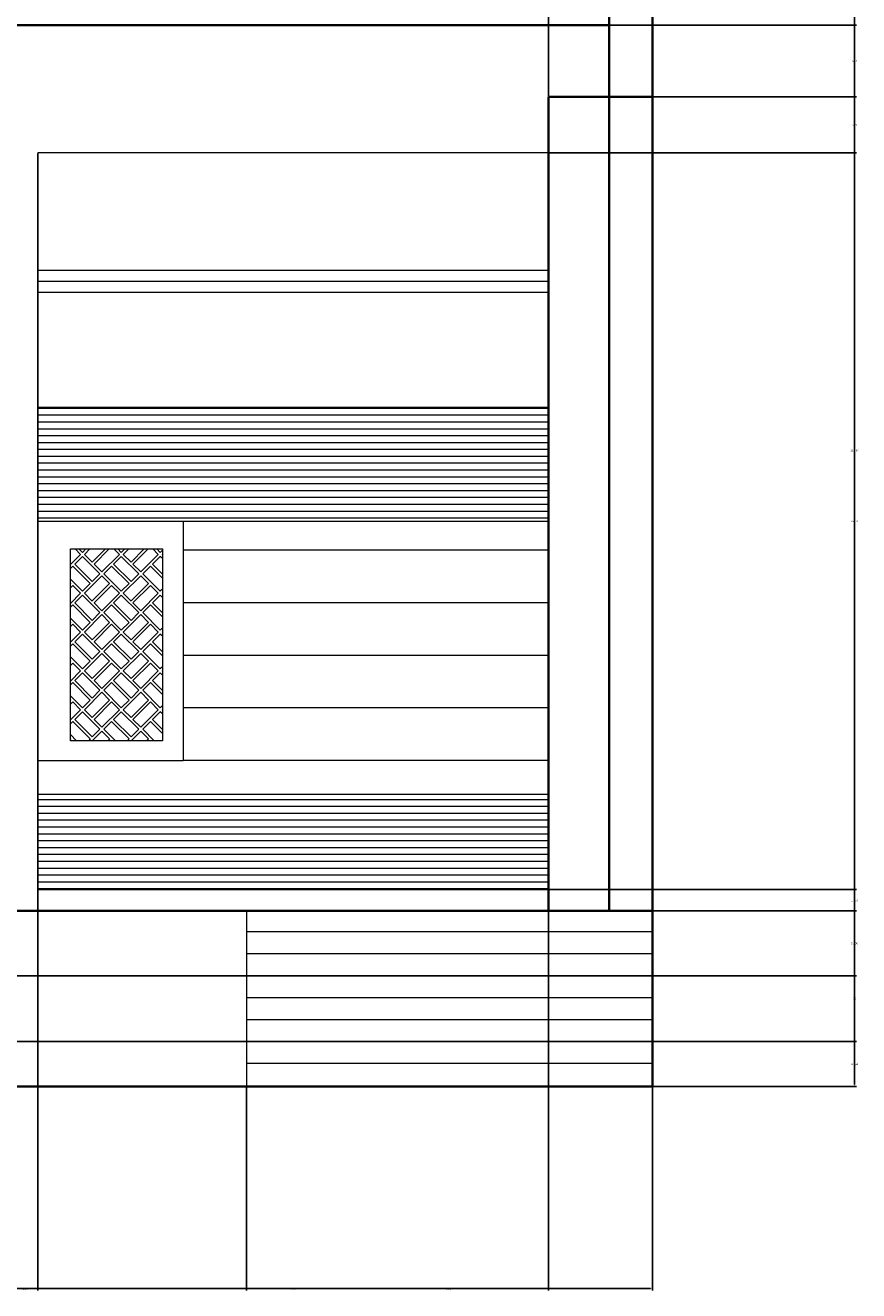
# Model space of a CAD drawing. Units: inches. Extents: x -7 to 391, y -12 to 303.
# Tile 4 of 5: x 315 to 391, y -12 to 103. Entities that reach past the tile are written whole.
import ezdxf

# ---------------------------------------------------------------- set-up
doc = ezdxf.new("R2010")
doc.units = ezdxf.units.IN
doc.header["$MEASUREMENT"] = 0
for name, color, linetype, lineweight in [('A-ANNO-DIMS', 2, 'Continuous', 18), ('A-DOOR', 3, 'Continuous', 18), ('A-ELEV', 7, 'Continuous', 35), ('A-ELEV-PATT', 8, 'Continuous', 13), ('A-FLOR-STRS', 2, 'Continuous', 18)]:
    doc.layers.add(name, color=color, linetype=linetype, lineweight=lineweight)
doc.styles.get("Standard").update_dxf_attribs({"font": 'arial.ttf'})
doc.dimstyles.get("Standard").update_dxf_attribs({"dimtxt": 0.18, "dimasz": 0.18, "dimexe": 0.18, "dimexo": 0.0625, "dimgap": 0.09, "dimtad": 0, "dimtih": 1, "dimtoh": 1, "dimdec": 4, "dimzin": 0, "dimdsep": 46, "dimtxsty": 'Standard', "dimcen": 0.09, "dimadec": 0, "dimazin": 0, "dimtfac": 1, "dimtdec": 4, "dimtofl": 0, "dimtmove": 0, "dimatfit": 3, "dimfxl": 1, "dimtolj": 1, "dimtzin": 0, "dimarcsym": 0})

# ---------------------------------------------------------------- blocks, each defined once
blk = doc.blocks.new('*D1')
at = {"layer": 'A-ANNO-DIMS', "color": 0, "lineweight": -2, "transparency": 16777216}
for p, q in [((372.08, 122.18), (390.6, 122.18)), ((390.42, 122), (390.42, 64.44)), ((390.42, 6.53), (390.42, 64.08)), ((150.31, 6.35), (390.6, 6.35))]:
    blk.add_line(p, q, dxfattribs=at)
at = {"layer": 'A-ANNO-DIMS', "color": 0, "transparency": 16777216}
for points in [[(390.39, 122), (390.45, 122), (390.42, 122.18)], [(390.39, 6.53), (390.45, 6.53), (390.42, 6.35)]]:
    blk.add_solid(points, dxfattribs=at)
at = {"layer": 'Defpoints', "color": 0, "transparency": 16777216}
for p in [(372.02, 122.18), (390.42, 122.18), (150.24, 6.35)]:
    blk.add_point(p, dxfattribs=at)
at = {"layer": 'A-ANNO-DIMS', "color": 0, "transparency": 16777216, "insert": (390.42, 64.26), "char_height": 0.18, "attachment_point": 5}
blk.add_mtext('\\A1;115.83', dxfattribs=at)
blk = doc.blocks.new('*D39')
at = {"layer": 'A-ANNO-DIMS', "color": 0, "lineweight": -2, "transparency": 16777216}
for p, q in [((372.02, 154.28), (372.02, -12.23)), ((246.74, 6.28), (246.74, -12.23)), ((246.92, -12.05), (308.92, -12.05)), ((371.84, -12.05), (309.84, -12.05))]:
    blk.add_line(p, q, dxfattribs=at)
at = {"layer": 'A-ANNO-DIMS', "color": 0, "transparency": 16777216}
for points in [[(246.92, -12.02), (246.92, -12.08), (246.74, -12.05)], [(371.84, -12.02), (371.84, -12.08), (372.02, -12.05)]]:
    blk.add_solid(points, dxfattribs=at)
at = {"layer": 'Defpoints', "color": 0, "transparency": 16777216}
for p in [(372.02, 154.35), (246.74, 6.35), (372.02, -12.05)]:
    blk.add_point(p, dxfattribs=at)
at = {"layer": 'A-ANNO-DIMS', "color": 0, "transparency": 16777216, "insert": (309.38, -12.05), "char_height": 0.18, "attachment_point": 5}
blk.add_mtext('\\A1;125.28', dxfattribs=at)
blk = doc.blocks.new('*D41')
at = {"layer": 'A-ANNO-DIMS', "color": 0, "lineweight": -2, "transparency": 16777216}
for p, q in [((283.68, 6.28), (283.68, -12.23)), ((335.08, 6.28), (335.08, -12.23)), ((283.86, -12.05), (309.06, -12.05)), ((334.9, -12.05), (309.7, -12.05))]:
    blk.add_line(p, q, dxfattribs=at)
at = {"layer": 'A-ANNO-DIMS', "color": 0, "transparency": 16777216}
for points in [[(283.86, -12.02), (283.86, -12.08), (283.68, -12.05)], [(334.9, -12.02), (334.9, -12.08), (335.08, -12.05)]]:
    blk.add_solid(points, dxfattribs=at)
at = {"layer": 'Defpoints', "color": 0, "transparency": 16777216}
for p in [(283.68, 6.35), (335.08, 6.35), (335.08, -12.05)]:
    blk.add_point(p, dxfattribs=at)
at = {"layer": 'A-ANNO-DIMS', "color": 0, "transparency": 16777216, "insert": (309.38, -12.05), "char_height": 0.18, "attachment_point": 5}
blk.add_mtext('\\A1;51.4', dxfattribs=at)
blk = doc.blocks.new('*D42')
at = {"layer": 'A-ANNO-DIMS', "color": 0, "lineweight": -2, "transparency": 16777216}
for p, q in [((335.08, 6.28), (335.08, -12.23)), ((372.02, 6.28), (372.02, -12.23)), ((335.26, -12.05), (353.16, -12.05)), ((371.84, -12.05), (353.94, -12.05))]:
    blk.add_line(p, q, dxfattribs=at)
at = {"layer": 'A-ANNO-DIMS', "color": 0, "transparency": 16777216}
for points in [[(335.26, -12.02), (335.26, -12.08), (335.08, -12.05)], [(371.84, -12.02), (371.84, -12.08), (372.02, -12.05)]]:
    blk.add_solid(points, dxfattribs=at)
at = {"layer": 'Defpoints', "color": 0, "transparency": 16777216}
for p in [(335.08, 6.35), (372.02, 6.35), (372.02, -12.05)]:
    blk.add_point(p, dxfattribs=at)
at = {"layer": 'A-ANNO-DIMS', "color": 0, "transparency": 16777216, "insert": (353.55, -12.05), "char_height": 0.18, "attachment_point": 5}
blk.add_mtext('\\A1;36.94', dxfattribs=at)
blk = doc.blocks.new('*D49')
at = {"layer": 'A-ANNO-DIMS', "color": 0, "lineweight": -2, "transparency": 16777216}
for p, q in [((313.81, 91.3), (313.81, -12.23)), ((316.08, 91.3), (316.08, -12.23)), ((313.99, -12.05), (314.62, -12.05)), ((315.9, -12.05), (315.27, -12.05))]:
    blk.add_line(p, q, dxfattribs=at)
at = {"layer": 'A-ANNO-DIMS', "color": 0, "transparency": 16777216}
for points in [[(313.99, -12.02), (313.99, -12.08), (313.81, -12.05)], [(315.9, -12.02), (315.9, -12.08), (316.08, -12.05)]]:
    blk.add_solid(points, dxfattribs=at)
at = {"layer": 'Defpoints', "color": 0, "transparency": 16777216}
for p in [(313.81, 91.37), (316.08, 91.37), (316.08, -12.05)]:
    blk.add_point(p, dxfattribs=at)
at = {"layer": 'A-ANNO-DIMS', "color": 0, "transparency": 16777216, "insert": (314.94, -12.05), "char_height": 0.18, "attachment_point": 5}
blk.add_mtext('\\A1;2.27', dxfattribs=at)
blk = doc.blocks.new('*D50')
at = {"layer": 'A-ANNO-DIMS', "color": 0, "lineweight": -2, "transparency": 16777216}
for p, q in [((316.08, 91.3), (316.08, -12.23)), ((362.55, 91.3), (362.55, -12.23)), ((316.26, -12.05), (338.92, -12.05)), ((362.37, -12.05), (339.71, -12.05))]:
    blk.add_line(p, q, dxfattribs=at)
at = {"layer": 'A-ANNO-DIMS', "color": 0, "transparency": 16777216}
for points in [[(316.26, -12.02), (316.26, -12.08), (316.08, -12.05)], [(362.37, -12.02), (362.37, -12.08), (362.55, -12.05)]]:
    blk.add_solid(points, dxfattribs=at)
at = {"layer": 'Defpoints', "color": 0, "transparency": 16777216}
for p in [(316.08, 91.37), (362.55, 91.37), (362.55, -12.05)]:
    blk.add_point(p, dxfattribs=at)
at = {"layer": 'A-ANNO-DIMS', "color": 0, "transparency": 16777216, "insert": (339.31, -12.05), "char_height": 0.18, "attachment_point": 5}
blk.add_mtext('\\A1;46.47', dxfattribs=at)
blk = doc.blocks.new('*D51')
at = {"layer": 'A-ANNO-DIMS', "color": 0, "lineweight": -2, "transparency": 16777216}
for p, q in [((362.55, 96.52), (362.55, 303.01)), ((368.1, 103.04), (368.1, 303.01)), ((362.73, 302.83), (364.93, 302.83)), ((367.92, 302.83), (365.72, 302.83))]:
    blk.add_line(p, q, dxfattribs=at)
at = {"layer": 'A-ANNO-DIMS', "color": 0, "transparency": 16777216}
for points in [[(362.73, 302.86), (362.73, 302.8), (362.55, 302.83)], [(367.92, 302.86), (367.92, 302.8), (368.1, 302.83)]]:
    blk.add_solid(points, dxfattribs=at)
at = {"layer": 'Defpoints', "color": 0, "transparency": 16777216}
for p in [(368.1, 302.83), (368.1, 102.98), (362.55, 96.46)]:
    blk.add_point(p, dxfattribs=at)
at = {"layer": 'A-ANNO-DIMS', "color": 0, "transparency": 16777216, "insert": (365.32, 302.83), "char_height": 0.18, "attachment_point": 5}
blk.add_mtext('\\A1;5.549', dxfattribs=at)
blk = doc.blocks.new('*D57')
at = {"layer": 'A-ANNO-DIMS', "color": 0, "lineweight": -2, "transparency": 16777216}
for p, q in [((372.08, 22.35), (390.6, 22.35)), ((390.42, 22.17), (390.42, 14.53)), ((390.42, 6.53), (390.42, 14.16)), ((372.08, 6.35), (390.6, 6.35))]:
    blk.add_line(p, q, dxfattribs=at)
at = {"layer": 'A-ANNO-DIMS', "color": 0, "transparency": 16777216}
for points in [[(390.39, 22.17), (390.45, 22.17), (390.42, 22.35)], [(390.39, 6.53), (390.45, 6.53), (390.42, 6.35)]]:
    blk.add_solid(points, dxfattribs=at)
at = {"layer": 'Defpoints', "color": 0, "transparency": 16777216}
for p in [(372.02, 22.35), (390.42, 22.35), (372.02, 6.35)]:
    blk.add_point(p, dxfattribs=at)
at = {"layer": 'A-ANNO-DIMS', "color": 0, "transparency": 16777216, "insert": (390.42, 14.35), "char_height": 0.18, "attachment_point": 5}
blk.add_mtext('\\A1;16', dxfattribs=at)
blk = doc.blocks.new('*D58')
at = {"layer": 'A-ANNO-DIMS', "color": 0, "lineweight": -2, "transparency": 16777216}
for p, q in [((362.61, 24.3), (390.6, 24.3)), ((390.42, 24.12), (390.42, 23.5)), ((390.42, 22.53), (390.42, 23.14)), ((372.08, 22.35), (390.6, 22.35))]:
    blk.add_line(p, q, dxfattribs=at)
at = {"layer": 'A-ANNO-DIMS', "color": 0, "transparency": 16777216}
for points in [[(390.39, 24.12), (390.45, 24.12), (390.42, 24.3)], [(390.39, 22.53), (390.45, 22.53), (390.42, 22.35)]]:
    blk.add_solid(points, dxfattribs=at)
at = {"layer": 'Defpoints', "color": 0, "transparency": 16777216}
for p in [(362.55, 24.3), (390.42, 24.3), (372.02, 22.35)]:
    blk.add_point(p, dxfattribs=at)
at = {"layer": 'A-ANNO-DIMS', "color": 0, "transparency": 16777216, "insert": (390.42, 23.32), "char_height": 0.18, "attachment_point": 5}
blk.add_mtext('\\A1;1.952', dxfattribs=at)
blk = doc.blocks.new('*D59')
at = {"layer": 'A-ANNO-DIMS', "color": 0, "lineweight": -2, "transparency": 16777216}
for p, q in [((362.61, 91.37), (390.6, 91.37)), ((390.42, 91.19), (390.42, 58.01)), ((390.42, 24.48), (390.42, 57.65)), ((362.61, 24.3), (390.6, 24.3))]:
    blk.add_line(p, q, dxfattribs=at)
at = {"layer": 'A-ANNO-DIMS', "color": 0, "transparency": 16777216}
for points in [[(390.39, 91.19), (390.45, 91.19), (390.42, 91.37)], [(390.39, 24.48), (390.45, 24.48), (390.42, 24.3)]]:
    blk.add_solid(points, dxfattribs=at)
at = {"layer": 'Defpoints', "color": 0, "transparency": 16777216}
for p in [(362.55, 91.37), (390.42, 91.37), (362.55, 24.3)]:
    blk.add_point(p, dxfattribs=at)
at = {"layer": 'A-ANNO-DIMS', "color": 0, "transparency": 16777216, "insert": (390.42, 57.83), "char_height": 0.18, "attachment_point": 5}
blk.add_mtext('\\A1;67.07', dxfattribs=at)
blk = doc.blocks.new('*D60')
at = {"layer": 'A-ANNO-DIMS', "color": 0, "lineweight": -2, "transparency": 16777216}
for p, q in [((372.08, 96.46), (390.6, 96.46)), ((390.42, 96.28), (390.42, 94.09)), ((390.42, 91.55), (390.42, 93.73)), ((362.61, 91.37), (390.6, 91.37))]:
    blk.add_line(p, q, dxfattribs=at)
at = {"layer": 'A-ANNO-DIMS', "color": 0, "transparency": 16777216}
for points in [[(390.39, 96.28), (390.45, 96.28), (390.42, 96.46)], [(390.39, 91.55), (390.45, 91.55), (390.42, 91.37)]]:
    blk.add_solid(points, dxfattribs=at)
at = {"layer": 'Defpoints', "color": 0, "transparency": 16777216}
for p in [(372.02, 96.46), (390.42, 96.46), (362.55, 91.37)]:
    blk.add_point(p, dxfattribs=at)
at = {"layer": 'A-ANNO-DIMS', "color": 0, "transparency": 16777216, "insert": (390.42, 93.91), "char_height": 0.18, "attachment_point": 5}
blk.add_mtext('\\A1;5.09', dxfattribs=at)
blk = doc.blocks.new('*D61')
at = {"layer": 'A-ANNO-DIMS', "color": 0, "lineweight": -2, "transparency": 16777216}
for p, q in [((368.16, 102.98), (390.6, 102.98)), ((390.42, 102.8), (390.42, 99.9)), ((390.42, 96.64), (390.42, 99.53)), ((372.08, 96.46), (390.6, 96.46))]:
    blk.add_line(p, q, dxfattribs=at)
at = {"layer": 'A-ANNO-DIMS', "color": 0, "transparency": 16777216}
for points in [[(390.39, 102.8), (390.45, 102.8), (390.42, 102.98)], [(390.39, 96.64), (390.45, 96.64), (390.42, 96.46)]]:
    blk.add_solid(points, dxfattribs=at)
at = {"layer": 'Defpoints', "color": 0, "transparency": 16777216}
for p in [(368.1, 102.98), (390.42, 102.98), (372.02, 96.46)]:
    blk.add_point(p, dxfattribs=at)
at = {"layer": 'A-ANNO-DIMS', "color": 0, "transparency": 16777216, "insert": (390.42, 99.72), "char_height": 0.18, "attachment_point": 5}
blk.add_mtext('\\A1;6.52', dxfattribs=at)
blk = doc.blocks.new('*D74')
at = {"layer": 'A-ANNO-DIMS', "color": 0, "lineweight": -2, "transparency": 16777216}
for p, q in [((283.74, 10.44), (390.6, 10.44)), ((390.42, 10.26), (390.42, 8.57)), ((390.42, 6.53), (390.42, 8.21)), ((283.74, 6.35), (390.6, 6.35))]:
    blk.add_line(p, q, dxfattribs=at)
at = {"layer": 'A-ANNO-DIMS', "color": 0, "transparency": 16777216}
for points in [[(390.39, 10.26), (390.45, 10.26), (390.42, 10.44)], [(390.39, 6.53), (390.45, 6.53), (390.42, 6.35)]]:
    blk.add_solid(points, dxfattribs=at)
at = {"layer": 'Defpoints', "color": 0, "transparency": 16777216}
for p in [(283.68, 10.44), (390.42, 10.44), (283.68, 6.35)]:
    blk.add_point(p, dxfattribs=at)
at = {"layer": 'A-ANNO-DIMS', "color": 0, "transparency": 16777216, "insert": (390.42, 8.39), "char_height": 0.18, "attachment_point": 5}
blk.add_mtext('\\A1;4.094', dxfattribs=at)
blk = doc.blocks.new('*D75')
at = {"layer": 'A-ANNO-DIMS', "color": 0, "lineweight": -2, "transparency": 16777216}
for p, q in [((283.74, 16.44), (390.6, 16.44)), ((390.42, 16.26), (390.42, 13.62)), ((390.42, 10.62), (390.42, 13.26)), ((283.74, 10.44), (390.6, 10.44))]:
    blk.add_line(p, q, dxfattribs=at)
at = {"layer": 'A-ANNO-DIMS', "color": 0, "transparency": 16777216}
for points in [[(390.39, 16.26), (390.45, 16.26), (390.42, 16.44)], [(390.39, 10.62), (390.45, 10.62), (390.42, 10.44)]]:
    blk.add_solid(points, dxfattribs=at)
at = {"layer": 'Defpoints', "color": 0, "transparency": 16777216}
for p in [(283.68, 16.44), (390.42, 16.44), (283.68, 10.44)]:
    blk.add_point(p, dxfattribs=at)
at = {"layer": 'A-ANNO-DIMS', "color": 0, "transparency": 16777216, "insert": (390.42, 13.44), "char_height": 0.18, "attachment_point": 5}
blk.add_mtext('\\A1;6', dxfattribs=at)
blk = doc.blocks.new('*D76')
at = {"layer": 'A-ANNO-DIMS', "color": 0, "lineweight": -2, "transparency": 16777216}
for p, q in [((283.74, 22.35), (390.6, 22.35)), ((390.42, 22.17), (390.42, 19.57)), ((390.42, 16.62), (390.42, 19.21)), ((283.74, 16.44), (390.6, 16.44))]:
    blk.add_line(p, q, dxfattribs=at)
at = {"layer": 'A-ANNO-DIMS', "color": 0, "transparency": 16777216}
for points in [[(390.39, 22.17), (390.45, 22.17), (390.42, 22.35)], [(390.39, 16.62), (390.45, 16.62), (390.42, 16.44)]]:
    blk.add_solid(points, dxfattribs=at)
at = {"layer": 'Defpoints', "color": 0, "transparency": 16777216}
for p in [(283.68, 22.35), (390.42, 22.35), (283.68, 16.44)]:
    blk.add_point(p, dxfattribs=at)
at = {"layer": 'A-ANNO-DIMS', "color": 0, "transparency": 16777216, "insert": (390.42, 19.39), "char_height": 0.18, "attachment_point": 5}
blk.add_mtext('\\A1;5.906', dxfattribs=at)

msp = doc.modelspace()

# ---------------------------------------------------------------- hatches: boundary and pattern name
at = {"layer": 'A-ELEV-PATT'}
h = msp.add_hatch(dxfattribs=at)
h.set_pattern_fill('ANSI31', color=256, scale=5, angle=135)
h.paths.add_polyline_path([(313.8105, 33.3417), (264.1332, 33.3417), (264.1332, 24.2974), (313.8105, 24.2974)])
h.paths.add_polyline_path([(362.5506, 32.9858), (316.076, 32.9858), (316.076, 24.2974), (362.5506, 24.2974)])
h.paths.add_polyline_path([(362.5506, 68.2193), (316.076, 68.2193), (316.076, 57.8315), (329.3009, 57.8315), (362.5506, 57.8315)])
h.paths.add_polyline_path([(313.8105, 68.2193), (264.1332, 68.2193), (264.1332, 57.8315), (313.8105, 57.8315)])
h = msp.add_hatch(dxfattribs=at)
h.set_pattern_fill('2X2µØ×©', color=256, scale=5, angle=135)
h.set_pattern_definition([(135, (0, 0), (-3.535534, 2e-16), [2.25, -0.25, 1, -0.25, 1, -0.25]), (135, (-0.707, -0.707), (-3.535534, 2e-16), [2.25, -2.75]), (135, (-0.884, -0.884), (-3.535534, 2e-16), [2.25, -2.75]), (135, (-1.591, -1.591), (-3.535534, 2e-16), [2.25, -0.25, 1, -0.25, 1, -0.25]), (225, (0, 0), (-4e-16, -3.535534), [1, -0.25, 1, -0.25, 2.25, -0.25]), (225, (-1.591, 1.591), (-4e-16, -3.535534), [1, -0.25, 1, -0.25, 2.25, -0.25]), (225, (-2.4749, 2.4749), (-4e-16, -3.535534), [2.25, -2.75]), (225, (-2.6517, 2.6517), (-4e-16, -3.535534), [2.25, -2.75])])
h.paths.add_polyline_path([(275.4815, 55.2969), (267.1041, 55.2969), (267.1041, 37.8416), (275.4815, 37.8416)])
h.paths.add_polyline_path([(327.4242, 55.2969), (319.0469, 55.2969), (319.0469, 37.8416), (327.4242, 37.8416)])

# ---------------------------------------------------------------- linework, layer by layer
at = {"layer": 'A-DOOR'}
for p, q in [((316.076, 80.6934), (362.5506, 80.6934)), ((316.076, 79.6934), (362.5506, 79.6934)), ((316.076, 79.6934), (362.5506, 79.6934)), ((316.076, 78.6934), (362.5506, 78.6934)), ((316.076, 68.2193), (362.5506, 68.2193)), ((316.076, 57.8315), (362.5506, 57.8315)), ((329.3009, 55.2077), (362.5506, 55.2077)), ((329.3009, 50.4241), (362.5506, 50.4241)), ((329.3009, 45.6405), (362.5506, 45.6405)), ((329.3009, 40.8569), (362.5506, 40.8569)), ((329.3009, 36.0733), (362.5506, 36.0733)), ((316.076, 32.9858), (362.5506, 32.9858))]:
    msp.add_line(p, q, dxfattribs=at)
for points in [[(362.5506, 91.3657), (316.076, 91.3657), (316.076, 24.2974), (362.5506, 24.2974)], [(316.076, 57.8315), (329.3009, 57.8315), (329.3009, 36.0134), (316.076, 36.0134)], [(319.0469, 55.2969), (327.4242, 55.2969), (327.4242, 37.8416), (319.0469, 37.8416)]]:
    msp.add_lwpolyline(points, close=True, dxfattribs=at)
at = {"layer": 'A-ELEV'}
for p, q in [((372.0212, 135.1767), (372.0212, 6.3452)), ((368.0993, 96.456), (368.0993, 122.1767)), ((258.2707, 102.9762), (368.0993, 102.9762)), ((362.5506, 22.3452), (362.5506, 96.456)), ((362.5506, 96.456), (368.0993, 96.456)), ((368.0993, 22.3452), (368.0993, 96.456)), ((368.0993, 96.456), (372.0212, 96.456)), ((12.0212, 22.3452), (372.0212, 22.3452)), ((12.0212, 6.3452), (372.0212, 6.3452))]:
    msp.add_line(p, q, dxfattribs=at)
at = {"layer": 'A-FLOR-STRS'}
for p, q in [((335.0799, 22.3452), (335.0799, 6.3452)), ((372.0212, 20.4396), (335.0799, 20.4396)), ((372.0212, 18.4396), (335.0799, 18.4396)), ((283.6807, 16.4396), (335.0799, 16.4396)), ((372.0212, 16.4396), (335.0799, 16.4396)), ((372.0212, 14.4396), (335.0799, 14.4396)), ((372.0212, 12.4396), (335.0799, 12.4396)), ((283.6807, 10.4396), (335.0799, 10.4396)), ((372.0212, 10.4396), (335.0799, 10.4396)), ((372.0212, 8.4396), (335.0799, 8.4396))]:
    msp.add_line(p, q, dxfattribs=at)

# ---------------------------------------------------------------- dimensions: what is measured, and where the dimension line sits
at = {"layer": 'A-ANNO-DIMS'}
for base, p1, p2, override, picture, middle in [((368.0993, 302.832), (362.5506, 96.456), (368.0993, 102.9762), {"dimdec": 3, "dimlfac": 1, "dimrnd": 0, "dimzin": 0, "dimdsep": 46, "dimlunit": 2}, '*D51', (365.325, 302.832)), ((372.0212, -12.0548), (246.7395, 6.3452), (372.0212, 154.3452), {"dimdec": 2, "dimlfac": 1, "dimrnd": 0, "dimzin": 0, "dimdsep": 46, "dimlunit": 2}, '*D39', (309.3803, -12.0548)), ((316.076, -12.0548), (313.8105, 91.3657), (316.076, 91.3657), {"dimdec": 2, "dimlfac": 1, "dimrnd": 0, "dimzin": 0, "dimdsep": 46, "dimlunit": 2}, '*D49', (314.9432, -12.0548)), ((362.5506, -12.0548), (316.076, 91.3657), (362.5506, 91.3657), {"dimdec": 2, "dimlfac": 1, "dimrnd": 0, "dimzin": 0, "dimdsep": 46, "dimlunit": 2}, '*D50', (339.3133, -12.0548)), ((335.0799, -12.0548), (283.6807, 6.3452), (335.0799, 6.3452), {"dimdec": 1, "dimlfac": 1, "dimrnd": 0, "dimzin": 0, "dimdsep": 46, "dimlunit": 2}, '*D41', (309.3803, -12.0548)), ((372.0212, -12.0548), (335.0799, 6.3452), (372.0212, 6.3452), {"dimdec": 2, "dimlfac": 1, "dimrnd": 0, "dimzin": 0, "dimdsep": 46, "dimlunit": 2}, '*D42', (353.5506, -12.0548))]:
    dim = msp.add_linear_dim(base=base, p1=p1, p2=p2, dimstyle='Standard', override=override, dxfattribs=at)
    dim.commit()
    dim.dimension.update_dxf_attribs({"geometry": picture, "text_midpoint": middle})
for base, p1, p2, override, picture, middle in [((390.4212, 122.1767), (150.2426, 6.3452), (372.0212, 122.1767), {"dimdec": 2, "dimlfac": 1, "dimrnd": 0, "dimzin": 0, "dimdsep": 46, "dimlunit": 2}, '*D1', (390.4212, 64.261)), ((390.4212, 102.9762), (372.0212, 96.456), (368.0993, 102.9762), {"dimdec": 2, "dimlfac": 1, "dimrnd": 0, "dimzin": 0, "dimdsep": 46, "dimlunit": 2}, '*D61', (390.4212, 99.7161)), ((390.4212, 96.456), (362.5506, 91.3657), (372.0212, 96.456), {"dimdec": 2, "dimlfac": 1, "dimrnd": 0, "dimzin": 0, "dimdsep": 46, "dimlunit": 2}, '*D60', (390.4212, 93.9109)), ((390.4212, 91.3657), (362.5506, 24.2974), (362.5506, 91.3657), {"dimdec": 2, "dimlfac": 1, "dimrnd": 0, "dimzin": 0, "dimdsep": 46, "dimlunit": 2}, '*D59', (390.4212, 57.8315)), ((390.4212, 24.2974), (372.0212, 22.3452), (362.5506, 24.2974), {"dimdec": 3, "dimlfac": 1, "dimrnd": 0, "dimzin": 0, "dimdsep": 46, "dimlunit": 2}, '*D58', (390.4212, 23.3213)), ((390.4212, 22.3452), (283.6807, 16.4396), (283.6807, 22.3452), {"dimdec": 3, "dimlfac": 1, "dimrnd": 0, "dimzin": 0, "dimdsep": 46, "dimlunit": 2}, '*D76', (390.4212, 19.3924)), ((390.4212, 22.3452), (372.0212, 6.3452), (372.0212, 22.3452), {"dimdec": 0, "dimlfac": 1, "dimrnd": 0, "dimzin": 0, "dimdsep": 46, "dimlunit": 2}, '*D57', (390.4212, 14.3452)), ((390.4212, 16.4396), (283.6807, 10.4396), (283.6807, 16.4396), {"dimdec": 0, "dimlfac": 1, "dimrnd": 0, "dimzin": 0, "dimdsep": 46, "dimlunit": 2}, '*D75', (390.4212, 13.4396)), ((390.4212, 10.4396), (283.6807, 6.3452), (283.6807, 10.4396), {"dimdec": 3, "dimlfac": 1, "dimrnd": 0, "dimzin": 0, "dimdsep": 46, "dimlunit": 2}, '*D74', (390.4212, 8.3924))]:
    dim = msp.add_linear_dim(base=base, p1=p1, p2=p2, angle=90, dimstyle='Standard', override=override, dxfattribs=at)
    dim.commit()
    dim.dimension.update_dxf_attribs({"geometry": picture, "text_midpoint": middle})

doc.saveas('drawing.dxf')
